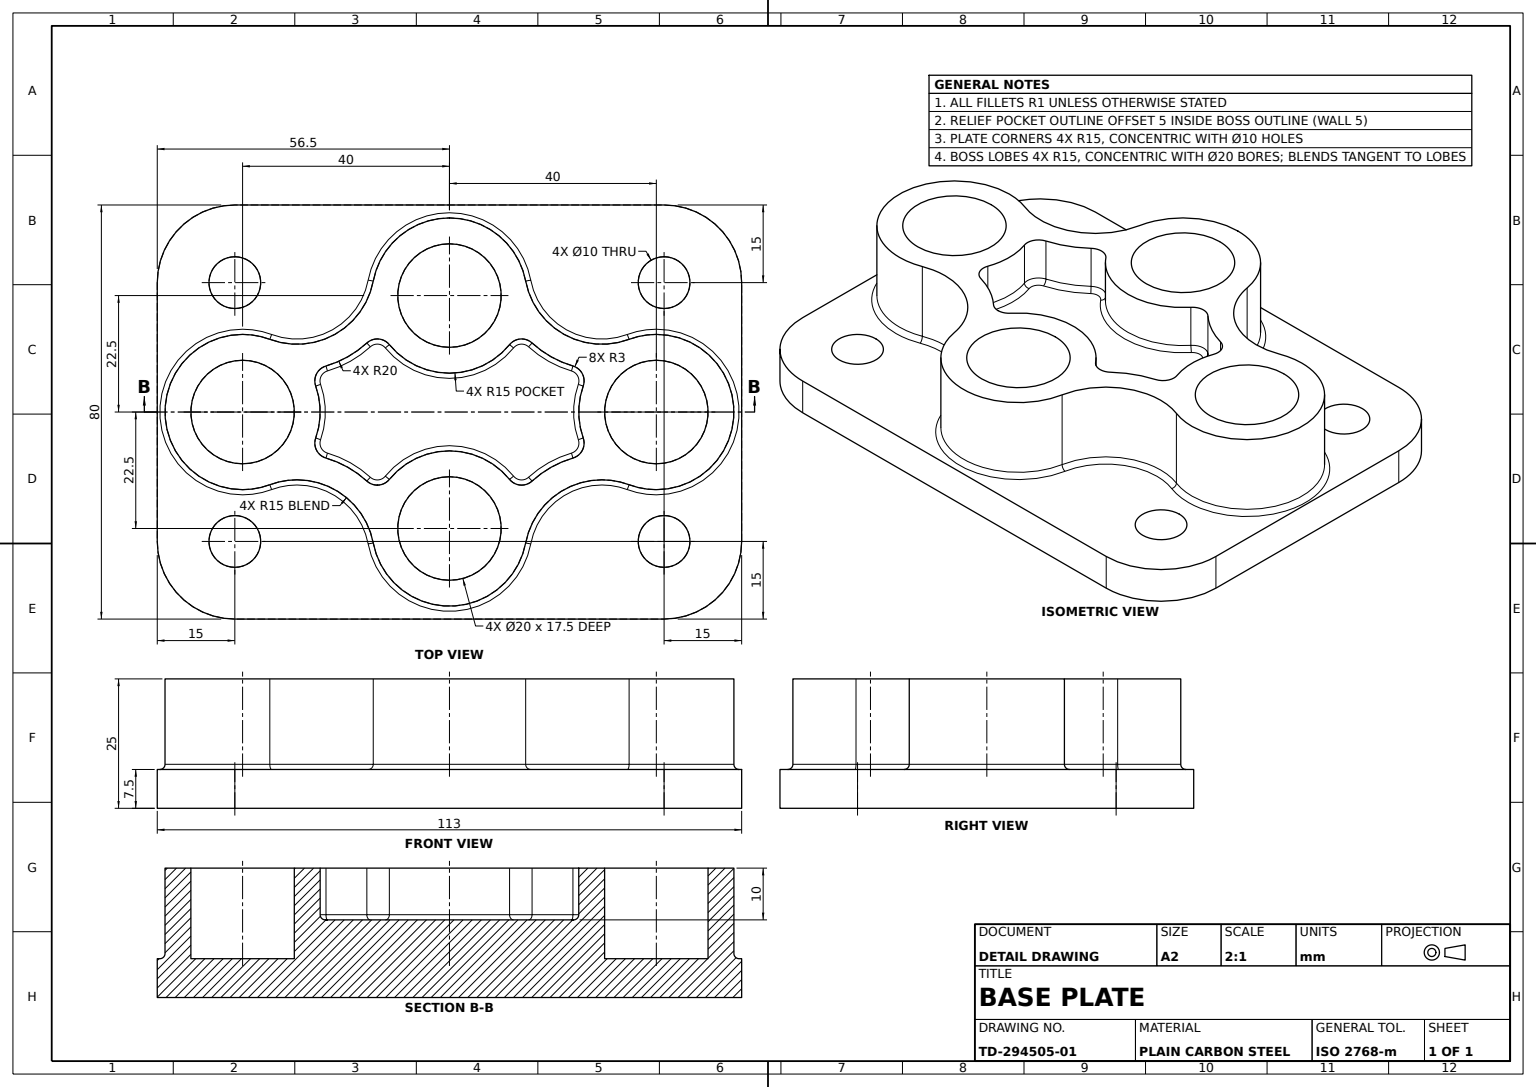
from build123d import *

# Parameters (mm, degrees)
BASE_PLATE_SKETCH_W              = 113
BASE_PLATE_SKETCH_H              = 80
BASE_PLATE_113X80X7_5_DEPTH      = 7.5
PLATE_CORNER_FILLETS_R15_R       = 15
MOUNTING_HOLES_SKETCH_R          = 5
CORNER_MOUNTING_HOLES_4X_DEPTH   = 7.5
BORE_BOSS_CLUSTER_SKETCH_R       = 10
BORE_BOSS_CLUSTER_DEPTH          = 17.5
BORES_START                      = -10
BORES_AND_RELIEF_POCKET_DEPTH    = 10
BOSS_ROOT_FILLET_R1_R            = 1
BORE_AND_POCKET_EDGE_FILLET_R1_R = 1


with BuildPart() as part:
    # Base Plate Sketch → Base Plate 113x80x7.5 (new body)
    with BuildSketch(Plane(origin=(0, 0, 0), x_dir=(1, 0, 0), z_dir=(0, 1, 0))):
        Rectangle(BASE_PLATE_SKETCH_W, BASE_PLATE_SKETCH_H)
    extrude(amount=BASE_PLATE_113X80X7_5_DEPTH)

    # Plate Corner Fillets R15
    plate_corner_fillets_r15_edges = [part.edges().sort_by_distance(p)[0] for p in [
        (56.5, 3.75, 40),
        (-56.5, 3.75, 40),
        (-56.5, 3.75, -40),
        (56.5, 3.75, -40),
    ]]
    fillet(plate_corner_fillets_r15_edges, radius=PLATE_CORNER_FILLETS_R15_R)

    # Mounting Holes Sketch → Corner Mounting Holes 4x (cut)
    with BuildSketch(Plane(origin=(0, 7.5, 0), x_dir=(1, 0, 0), z_dir=(0, 1, 0))):
        with Locations(Location((-41.5, 25, 0), (0, 0, 270))):
            Circle(MOUNTING_HOLES_SKETCH_R)
        with Locations(Location((41.5, 25, 0), (0, 0, 270))):
            Circle(MOUNTING_HOLES_SKETCH_R)
        with Locations(Location((-41.5, -25, 0), (0, 0, 270))):
            Circle(MOUNTING_HOLES_SKETCH_R)
        with Locations(Location((41.5, -25, 0), (0, 0, 270))):
            Circle(MOUNTING_HOLES_SKETCH_R)
    extrude(amount=-CORNER_MOUNTING_HOLES_4X_DEPTH, mode=Mode.SUBTRACT)

    # Bore Boss Cluster Sketch → Bore Boss Cluster (add)
    with BuildSketch(Plane(origin=(0, 7.5, 0), x_dir=(1, 0, 0), z_dir=(0, 1, 0))):
        with BuildLine():
            ThreePointArc((-34.737034272, 14.046394261), (-55, 0), (-34.737034272, -14.046394261))
            ThreePointArc((-34.737034272, -14.046394261), (-22.12014995, -15.019155466), (-14.737034272, -25.296394261))
            ThreePointArc((-14.737034272, -25.296394261), (0, -37.5), (14.737034272, -25.296394261))
            ThreePointArc((14.737034272, -25.296394261), (22.12014995, -15.019155466), (34.737034272, -14.046394261))
            ThreePointArc((34.737034272, -14.046394261), (55, 0), (34.737034272, 14.046394261))
            ThreePointArc((34.737034272, 14.046394261), (22.12014995, 15.019155466), (14.737034272, 25.296394261))
            ThreePointArc((14.737034272, 25.296394261), (0, 37.5), (-14.737034272, 25.296394261))
            ThreePointArc((-14.737034272, 25.296394261), (-22.12014995, 15.019155466), (-34.737034272, 14.046394261))
        make_face()
        with Locations(Location((-40, 0, 0), (0, 0, 270))):
            Circle(BORE_BOSS_CLUSTER_SKETCH_R, mode=Mode.SUBTRACT)
        with Locations(Location((0, 22.5, 0), (0, 0, 270))):
            Circle(BORE_BOSS_CLUSTER_SKETCH_R, mode=Mode.SUBTRACT)
        with Locations(Location((40, 0, 0), (0, 0, 270))):
            Circle(BORE_BOSS_CLUSTER_SKETCH_R, mode=Mode.SUBTRACT)
        with Locations(Location((0, -22.5, 0), (0, 0, 270))):
            Circle(BORE_BOSS_CLUSTER_SKETCH_R, mode=Mode.SUBTRACT)
    extrude(amount=BORE_BOSS_CLUSTER_DEPTH)

    # Bores and Relief Pocket Sketch → Bores and Relief Pocket (cut)
    with BuildSketch(Plane(origin=(0, 25, 0), x_dir=(1, 0, 0), z_dir=(0, 1, 0)).offset(BORES_START)):
        with BuildLine():
            ThreePointArc((-23.873986231, -8.892812531), (-25.704313442, -7.380034713), (-25.861644904, -5.01068011))
            ThreePointArc((-25.861644904, -5.01068011), (-25, 0), (-25.861644904, 5.01068011))
            ThreePointArc((-25.861644904, 5.01068011), (-25.704313442, 7.380034713), (-23.873986231, 8.892812531))
            ThreePointArc((-23.873986231, 8.892812531), (-19.668843751, 10.66127778), (-15.97383507, 13.336647559))
            ThreePointArc((-15.97383507, 13.336647559), (-13.730549392, 14.115276991), (-11.62400004, 13.019355346))
            ThreePointArc((-11.62400004, 13.019355346), (0, 7.5), (11.62400004, 13.019355346))
            ThreePointArc((11.62400004, 13.019355346), (13.730549392, 14.115276991), (15.97383507, 13.336647559))
            ThreePointArc((15.97383507, 13.336647559), (19.668843751, 10.66127778), (23.873986231, 8.892812531))
            ThreePointArc((23.873986231, 8.892812531), (25.704313442, 7.380034713), (25.861644904, 5.01068011))
            ThreePointArc((25.861644904, 5.01068011), (25, 0), (25.861644904, -5.01068011))
            ThreePointArc((25.861644904, -5.01068011), (25.704313442, -7.380034713), (23.873986231, -8.892812531))
            ThreePointArc((23.873986231, -8.892812531), (19.668843751, -10.66127778), (15.97383507, -13.336647559))
            ThreePointArc((15.97383507, -13.336647559), (13.730549392, -14.115276991), (11.62400004, -13.019355346))
            ThreePointArc((11.62400004, -13.019355346), (0, -7.5), (-11.62400004, -13.019355346))
            ThreePointArc((-11.62400004, -13.019355346), (-13.730549392, -14.115276991), (-15.97383507, -13.336647559))
            ThreePointArc((-15.97383507, -13.336647559), (-19.668843751, -10.66127778), (-23.873986231, -8.892812531))
        make_face()
    extrude(amount=BORES_AND_RELIEF_POCKET_DEPTH, mode=Mode.SUBTRACT)

    # Boss Root Fillet R1
    boss_root_fillet_r1_edges = [part.edges().sort_by_distance(p)[0] for p in [
        (-22.12014995, 7.5, -15.019155466),
        (-55, 7.5, 0),
        (-22.12014995, 7.5, 15.019155466),
        (0, 7.5, 37.5),
        (22.12014995, 7.5, 15.019155466),
        (55, 7.5, 0),
        (22.12014995, 7.5, -15.019155466),
        (0, 7.5, -37.5),
    ]]
    fillet(boss_root_fillet_r1_edges, radius=BOSS_ROOT_FILLET_R1_R)

    # Bore and Pocket Edge Fillet R1
    bore_and_pocket_edge_fillet_r1_edges = [part.edges().sort_by_distance(p)[0] for p in [
        (-19.668843751, 15, 10.66127778),
        (-25.704313442, 15, 7.380034713),
        (-25, 15, 0),
        (-25.704313442, 15, -7.380034713),
        (-19.668843751, 15, -10.66127778),
        (-13.730549392, 15, -14.115276991),
        (0, 15, -7.5),
        (13.730549392, 15, -14.115276991),
        (19.668843751, 15, -10.66127778),
        (25.704313442, 15, -7.380034713),
        (25, 15, 0),
        (25.704313442, 15, 7.380034713),
        (19.668843751, 15, 10.66127778),
        (13.730549392, 15, 14.115276991),
        (0, 15, 7.5),
        (-13.730549392, 15, 14.115276991),
    ]]
    fillet(bore_and_pocket_edge_fillet_r1_edges, radius=BORE_AND_POCKET_EDGE_FILLET_R1_R)


solid = part.part
